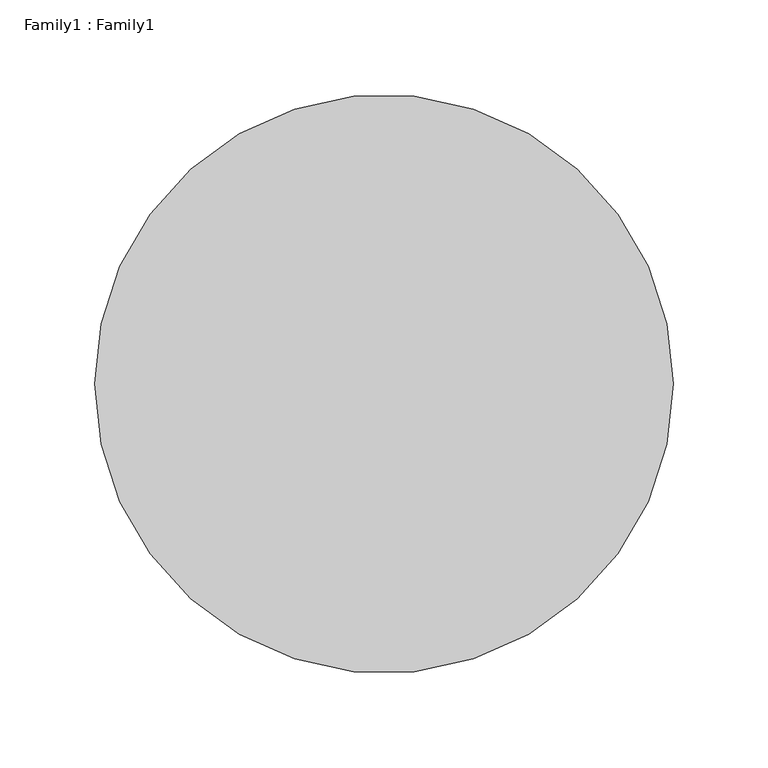
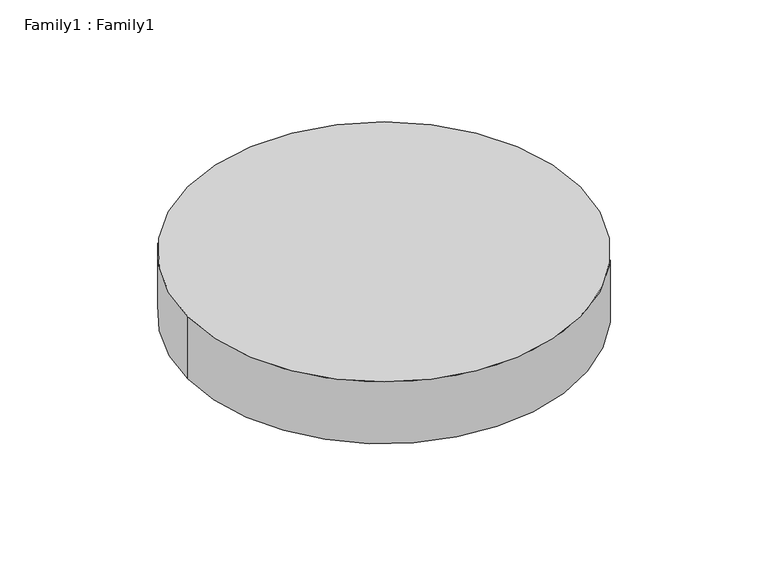
"""IFC4 building model written with IfcOpenShell, lengths in millimetres: light fixture geometry, Family1 : Family1."""

from ifc_helpers import new_model, si_unit, point, frame, origin, origin_2d, place, context, project, spatial, circle_curve, trimmed, segment, composite_curve, outline, extrude, source, transform, mapped, element, save


def family1_family1_bfb63c4d(model_context):
    return source(origin(), model_context, "Body", "SweptSolid", [
        extrude(outline(composite_curve([segment(trimmed(circle_curve(origin_2d(), 152.4), [point((-152.4, 0.0))], [point((152.4, 0.0))], False, "CARTESIAN"), True, "CONTINUOUS"), segment(trimmed(circle_curve(origin_2d(), 152.4), [point((152.4, 0.0))], [point((-152.4, 0.0))], False, "CARTESIAN"), True, "CONTINUOUS")], self_intersect=False)), frame((0.0, 0.0, 2438.4), z_axis=(0.0, 0.0, 1.0), x_axis=(1.0, 0.0, 0.0)), (0.0, 0.0, 1.0), 50.8),
    ])


if __name__ == "__main__":
    model = new_model("IFC4")
    model_context = context("Model", 3, world=origin())
    ifc_project = project(units=[si_unit("LENGTHUNIT", "METRE", prefix="MILLI")], contexts=[model_context])
    site = spatial("IfcSite", under=ifc_project)
    building = spatial("IfcBuilding", under=site)
    placement = place(None, origin())
    family1_family1_shape = family1_family1_bfb63c4d(model_context)
    element("IfcLightFixture", 1, ObjectType="Family1 : Family1", at=placement, inside=building, context=model_context, shape_type="MappedRepresentation", body=[
        mapped(family1_family1_shape, transform((0.0, 0.0, 0.0), x_axis=(1.0, 0.0, 0.0), y_axis=(0.0, 1.0, 0.0), z_axis=(0.0, 0.0, 1.0))),
    ])
    save(model, "model.ifc")

# Revit data of these elements
# Type "Family1 : Family1"
#   Photometric Web File = "generic"
#   Wattage = 12.1178 W
#   built-in parameter 1150110 = 1 (stored number, unit not read)
#   built-in parameter 1114217 = 1 (stored number, unit not read)
#   Tilt Angle = 60.00°
#   built-in parameter 1150109 = 1 (stored number, unit not read)
#   built-in parameter 1150113 = 1 (stored number, unit not read)
#   Lumens = 1800 lm
#   built-in parameter 1150115 = 1 (stored number, unit not read)
#   built-in parameter 1150105 = 143.239 (stored number, unit not read)
#   built-in parameter 1150112 = 1 (stored number, unit not read)
#   built-in parameter 1150114 = 1 (stored number, unit not read)
#   built-in parameter 1150107 = 3000 (stored number, unit not read)
#   built-in parameter 1150106 = 1.43239 (stored number, unit not read)
#   Emit from Circle Diameter = 2' - 0"
#   built-in parameter 1150104 = 13.8 (stored number, unit not read)
#   built-in parameter 1114218 = 1 (stored number, unit not read)
#   built-in parameter 1150133 = 10 (stored number, unit not read)
#   built-in parameter 1150132 = 2
#   Color Filter = 16777215
#   Emit Shape Visible in Rendering = no
#   Dimming Lamp Color Temperature Shift = (empty or 0)
#   Default Elevation = 0
